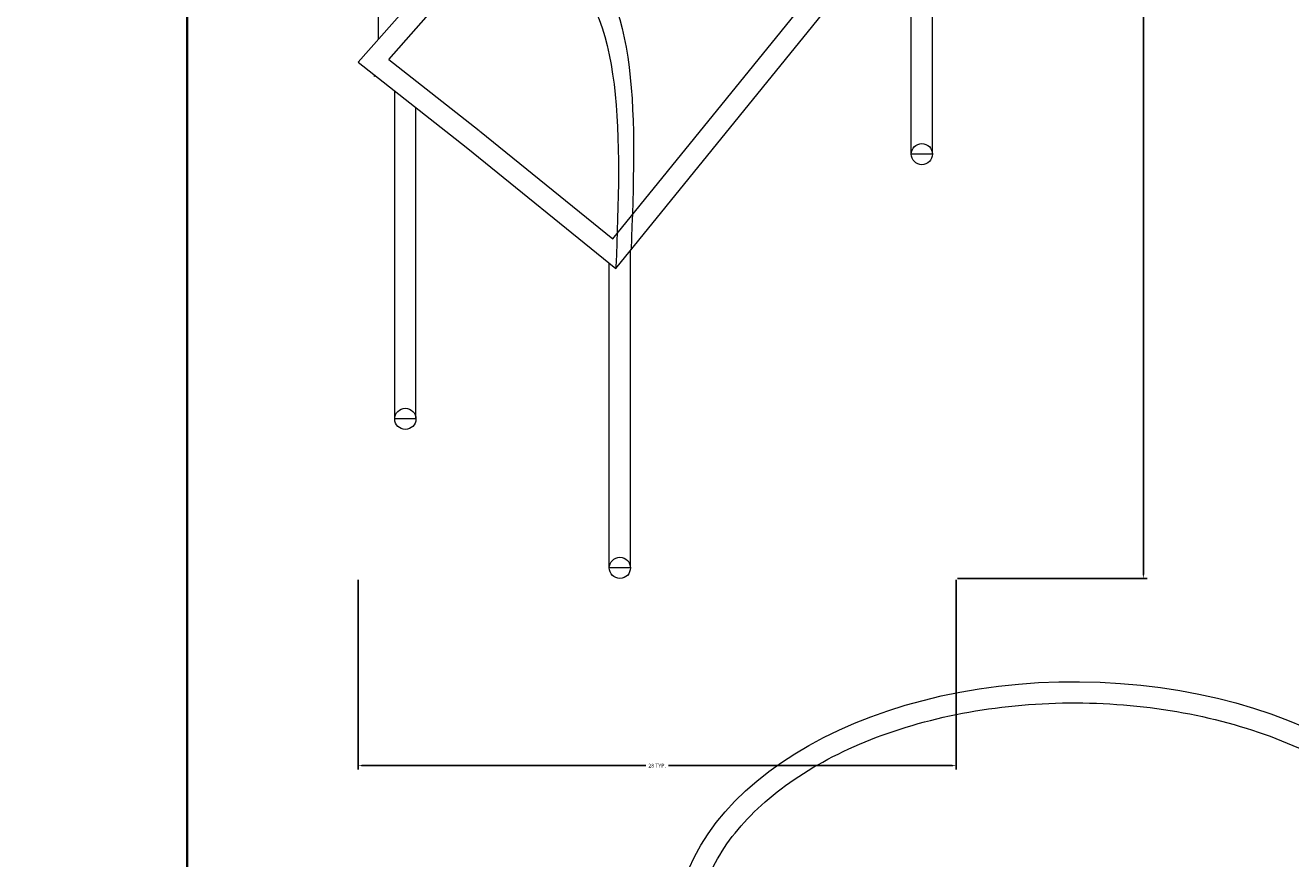
# Model space of a CAD drawing. Units: inches. Extents: x -61 to 1599, y -1316 to 257.
# Tile 16 of 204: x 16 to 76, y -868 to -829. Entities that reach past the tile are written whole.
import ezdxf

# ---------------------------------------------------------------- set-up
doc = ezdxf.new("R2010")
doc.units = ezdxf.units.IN
doc.header["$MEASUREMENT"] = 0
for name, color, linetype, lineweight in [('A-ANNO-DIMS', 2, 'Continuous', 18), ('FURNITURE', 83, 'Continuous', 18), ('WALLS', 4, 'Continuous', 35)]:
    doc.layers.add(name, color=color, linetype=linetype, lineweight=lineweight)
doc.styles.get("Standard").update_dxf_attribs({"font": 'arial.ttf'})
doc.dimstyles.get("Standard").update_dxf_attribs({"dimtxt": 0.18, "dimasz": 0.18, "dimexe": 0.18, "dimexo": 0.0625, "dimgap": 0.09, "dimtad": 0, "dimtih": 1, "dimtoh": 1, "dimdec": 0, "dimzin": 0, "dimdsep": 46, "dimlunit": 3, "dimtxsty": 'Standard', "dimcen": 0.09, "dimadec": 0, "dimazin": 0, "dimtfac": 1, "dimtdec": 0, "dimtofl": 0, "dimtmove": 0, "dimatfit": 3, "dimfxl": 1, "dimtolj": 1, "dimtzin": 0, "dimarcsym": 0})

# ---------------------------------------------------------------- blocks, each defined once
blk = doc.blocks.new('LOUNGE-CHAIR')
for p, q in [((0.966, 25.454), (0.966, 43.203)), ((0.966, 25.454), (0.966, 43.203)), ((0, 24.355), (16.378, 42.984)), ((1.449, 24.488), (16.505, 41.614)), ((12.015, 16.032), (26.35, 33.719)), ((12.162, 14.625), (27.757, 33.866)), ((27.098, 20.023), (27.098, 33.052)), ((26.098, 20.023), (26.098, 31.819)), ((1.449, 24.488), (5.717, 21.137)), ((0, 24.355), (5.099, 20.35)), ((0.751, 23.694), (0.787, 23.736)), ((1.726, 7.53), (1.726, 22.999)), ((2.726, 7.53), (2.726, 22.214)), ((5.729, 21.127), (12.015, 16.032)), ((5.099, 20.35), (12.162, 14.625)), ((27.098, 20.023), (26.098, 20.023)), ((12.851, 0.5), (12.851, 15.475)), ((11.851, 0.5), (11.851, 14.878)), ((2.726, 7.53), (1.726, 7.53)), ((12.851, 0.5), (11.851, 0.5))]:
    blk.add_line(p, q)
for centre in [(26.598, 20.023), (2.226, 7.53), (12.351, 0.5)]:
    blk.add_circle(centre, 0.5)
for points, knots in [([(1.64, 31.221), (4.989, 31.369), (13.472, 31.237), (13.106, 21.568), (12.877, 15.507)], [1.527723, 1.527723, 1.527723, 1.527723, 10.281855, 24.983674, 24.983674, 24.983674, 24.983674]), ([(1.64, 30.439), (4.722, 30.546), (12.751, 30.171), (12.394, 20.758), (12.165, 14.697), (12.164, 14.673), (12.163, 14.649), (12.162, 14.625)], [2.150702, 2.150702, 2.150702, 2.150702, 10.281855, 24.983674, 24.983674, 24.983674, 25.041855, 25.041855, 25.041855, 25.041855])]:
    blk.add_open_spline(points, degree=3, knots=knots)
blk = doc.blocks.new('SIDE-TABLE-OVAL')
blk.add_ellipse((18.952, 11.99), major_axis=(-18.953, 0.16), ratio=0.632617)
blk.add_open_spline([(1, 12.141), (0.991, 11.171), (1.197, 10.196), (2.048, 8.281), (2.695, 7.34), (4.411, 5.578), (5.479, 4.757), (7.957, 3.322), (9.367, 2.708), (12.412, 1.745), (14.047, 1.396), (17.407, 0.998), (19.132, 0.949), (22.53, 1.153), (24.202, 1.406), (27.357, 2.192), (28.839, 2.725), (31.489, 4.019), (32.657, 4.779), (34.59, 6.449), (35.353, 7.358), (36.437, 9.235), (36.759, 10.202), (36.972, 12.14), (36.865, 13.115), (36.215, 15.044), (35.67, 15.999), (34.148, 17.812), (33.171, 18.668), (30.853, 20.193), (29.513, 20.861), (26.577, 21.943), (24.982, 22.356), (21.67, 22.889), (19.953, 23.008), (16.539, 22.943), (14.842, 22.758), (11.607, 22.1), (10.07, 21.628), (7.283, 20.442), (6.033, 19.727), (3.921, 18.129), (3.059, 17.247), (1.775, 15.402), (1.352, 14.441), (1.052, 13.032), (1.003, 12.587), (1, 12.141)], degree=3, knots=[0, 0, 0, 0, 0.279765, 0.279765, 0.559529, 0.559529, 0.839294, 0.839294, 1.119059, 1.119059, 1.398823, 1.398823, 1.678588, 1.678588, 1.958353, 1.958353, 2.238118, 2.238118, 2.517882, 2.517882, 2.797647, 2.797647, 3.077412, 3.077412, 3.357176, 3.357176, 3.636941, 3.636941, 3.916706, 3.916706, 4.19647, 4.19647, 4.476235, 4.476235, 4.756, 4.756, 5.035764, 5.035764, 5.315529, 5.315529, 5.595294, 5.595294, 5.875058, 5.875058, 6.154823, 6.154823, 6.283185, 6.283185, 6.283185, 6.283185])
blk = doc.blocks.new('*D630')
at = {"layer": 'A-ANNO-DIMS', "color": 0, "lineweight": -2, "transparency": 16777216}
for p, q in [((60.054, -796.178), (69.005, -796.178)), ((68.825, -796.358), (68.825, -825.439)), ((68.825, -854.887), (68.825, -825.806)), ((60.054, -855.067), (69.005, -855.067))]:
    blk.add_line(p, q, dxfattribs=at)
at = {"layer": 'A-ANNO-DIMS', "color": 0, "transparency": 16777216}
for points in [[(68.795, -796.358), (68.855, -796.358), (68.825, -796.178)], [(68.795, -854.887), (68.855, -854.887), (68.825, -855.067)]]:
    blk.add_solid(points, dxfattribs=at)
at = {"layer": 'DEFPOINTS', "color": 0, "transparency": 16777216}
for p in [(59.992, -796.178), (68.825, -796.178), (59.992, -855.067)]:
    blk.add_point(p, dxfattribs=at)
at = {"layer": 'A-ANNO-DIMS', "color": 0, "transparency": 16777216, "insert": (68.825, -825.623), "char_height": 0.18, "attachment_point": 5}
blk.add_mtext('\\A1;LOUNGE CHAIR 59 TYP.', dxfattribs=at)
blk = doc.blocks.new('*D631')
at = {"layer": 'A-ANNO-DIMS', "color": 0, "lineweight": -2, "transparency": 16777216}
for p, q in [((31.776, -855.129), (31.776, -864.08)), ((59.992, -855.129), (59.992, -864.08)), ((31.956, -863.9), (45.354, -863.9)), ((59.812, -863.9), (46.413, -863.9))]:
    blk.add_line(p, q, dxfattribs=at)
at = {"layer": 'A-ANNO-DIMS', "color": 0, "transparency": 16777216}
for points in [[(31.956, -863.87), (31.956, -863.93), (31.776, -863.9)], [(59.812, -863.87), (59.812, -863.93), (59.992, -863.9)]]:
    blk.add_solid(points, dxfattribs=at)
at = {"layer": 'DEFPOINTS', "color": 0, "transparency": 16777216}
for p in [(31.776, -855.067), (59.992, -855.067), (59.992, -863.9)]:
    blk.add_point(p, dxfattribs=at)
at = {"layer": 'A-ANNO-DIMS', "color": 0, "transparency": 16777216, "insert": (45.884, -863.9), "char_height": 0.18, "attachment_point": 5}
blk.add_mtext('\\A1;28 TYP.', dxfattribs=at)
blk = doc.blocks.new('*D687')
at = {"layer": 'A-ANNO-DIMS', "color": 0, "lineweight": -2, "transparency": 16777216}
for p, q in [((289.418, 181.677), (-61.077, 181.677)), ((-60.897, 181.497), (-60.897, -528.952)), ((-60.897, -1239.765), (-60.897, -529.316)), ((319.64, -1239.945), (-61.077, -1239.945))]:
    blk.add_line(p, q, dxfattribs=at)
at = {"layer": 'A-ANNO-DIMS', "color": 0, "transparency": 16777216}
for points in [[(-60.927, 181.497), (-60.867, 181.497), (-60.897, 181.677)], [(-60.927, -1239.765), (-60.867, -1239.765), (-60.897, -1239.945)]]:
    blk.add_solid(points, dxfattribs=at)
at = {"layer": 'DEFPOINTS', "color": 0, "transparency": 16777216}
for p in [(289.481, 181.677), (-60.897, -1239.945), (319.703, -1239.945)]:
    blk.add_point(p, dxfattribs=at)
at = {"layer": 'A-ANNO-DIMS', "color": 0, "transparency": 16777216, "insert": (-60.897, -529.134), "char_height": 0.18, "attachment_point": 5}
blk.add_mtext('\\A1;1421.6', dxfattribs=at)

msp = doc.modelspace()

# ---------------------------------------------------------------- linework, layer by layer
at = {"layer": 'WALLS'}
msp.add_line((23.7028, -943.9446), (23.7028, -787.9446), dxfattribs=at)

# ---------------------------------------------------------------- block references
at = {"layer": 'FURNITURE'}
for name, p in [('LOUNGE-CHAIR', (31.776, -855.0667)), ('SIDE-TABLE-OVAL', (46.761, -883.9187))]:
    msp.add_blockref(name, p, dxfattribs=at)

# ---------------------------------------------------------------- dimensions: what is measured, and where the dimension line sits
at = {"layer": 'A-ANNO-DIMS'}
dim = msp.add_linear_dim(base=(-60.8972, -1239.9446), p1=(289.4807, 181.6771), p2=(319.7028, -1239.9446), angle=90, dimstyle='Standard', override={"dimdec": 1, "dimlfac": 1, "dimrnd": 0, "dimzin": 0, "dimdsep": 46, "dimlunit": 2}, dxfattribs=at)
dim.commit()
dim.dimension.update_dxf_attribs({"geometry": '*D687', "text_midpoint": (-60.8972, -529.1337)})
dim = msp.add_linear_dim(base=(68.825, -796.1784), p1=(59.9918, -855.0667), p2=(59.9918, -796.1784), angle=90, text='LOUNGE CHAIR <> TYP.', dimstyle='Standard', override={"dimdec": 0, "dimlfac": 1, "dimrnd": 0, "dimzin": 0, "dimdsep": 46, "dimlunit": 2}, dxfattribs=at)
dim.commit()
dim.dimension.update_dxf_attribs({"geometry": '*D630', "text_midpoint": (68.825, -825.6226)})
dim = msp.add_linear_dim(base=(59.9918, -863.8999), p1=(31.7756, -855.0667), p2=(59.9918, -855.0667), text='<> TYP.', dimstyle='Standard', override={"dimdec": 0, "dimlfac": 1, "dimrnd": 0, "dimzin": 0, "dimdsep": 46, "dimlunit": 2}, dxfattribs=at)
dim.commit()
dim.dimension.update_dxf_attribs({"geometry": '*D631', "text_midpoint": (45.8837, -863.8999)})

doc.saveas('drawing.dxf')
